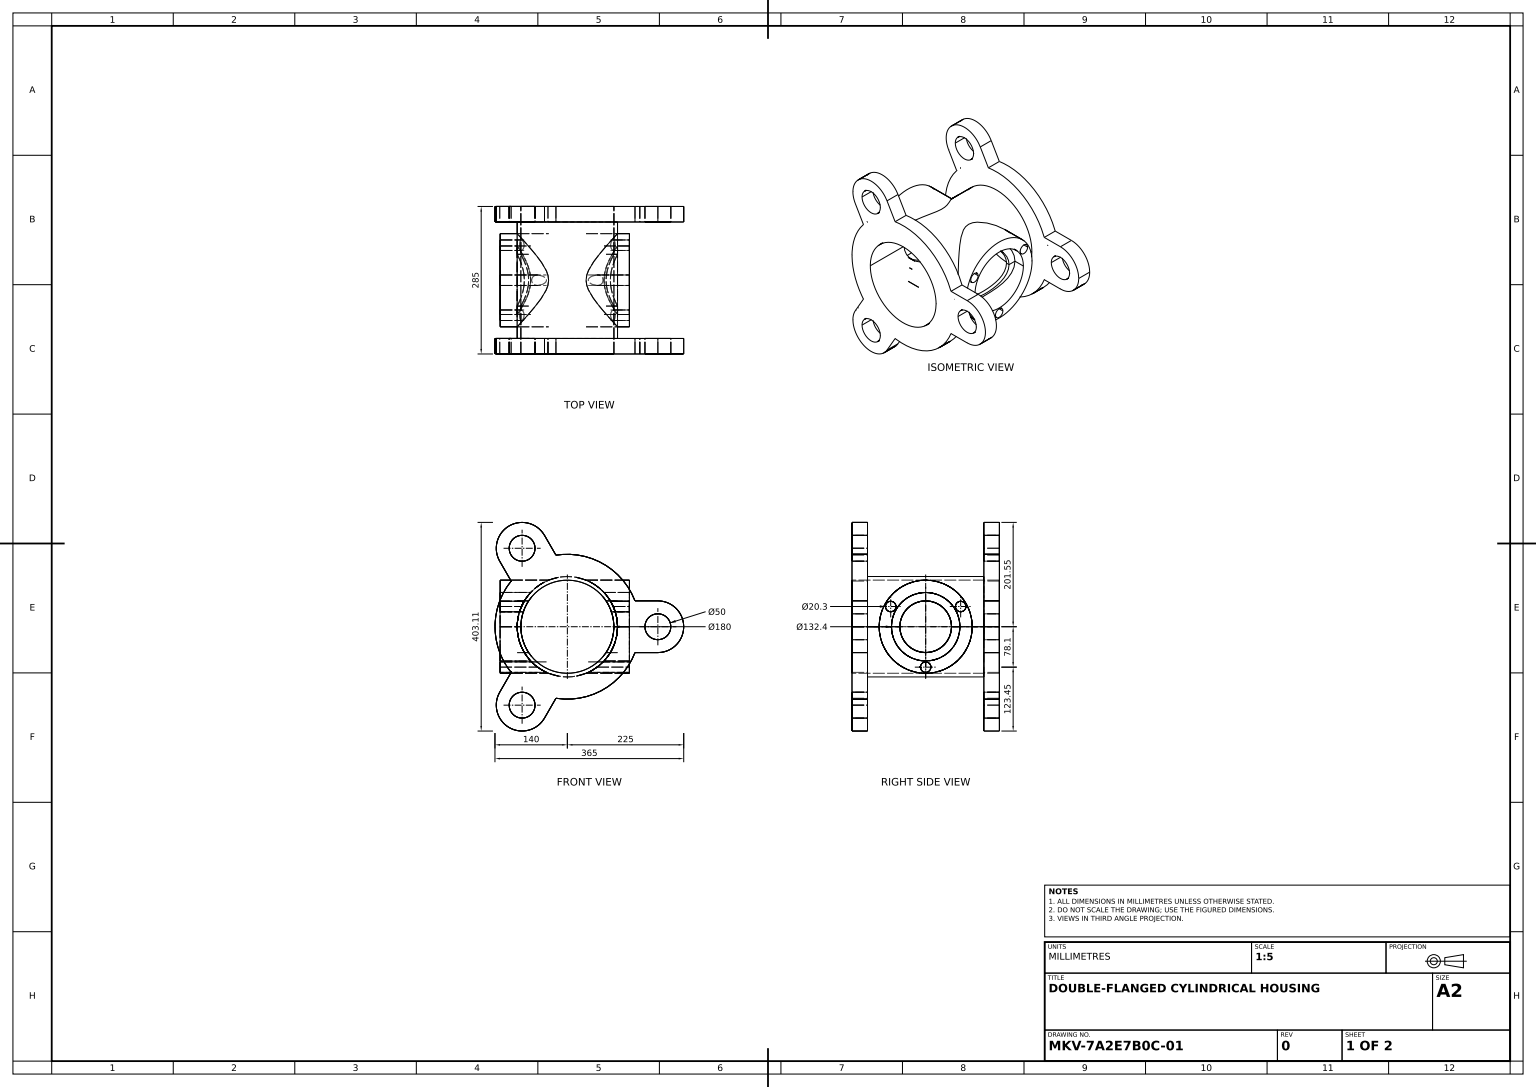
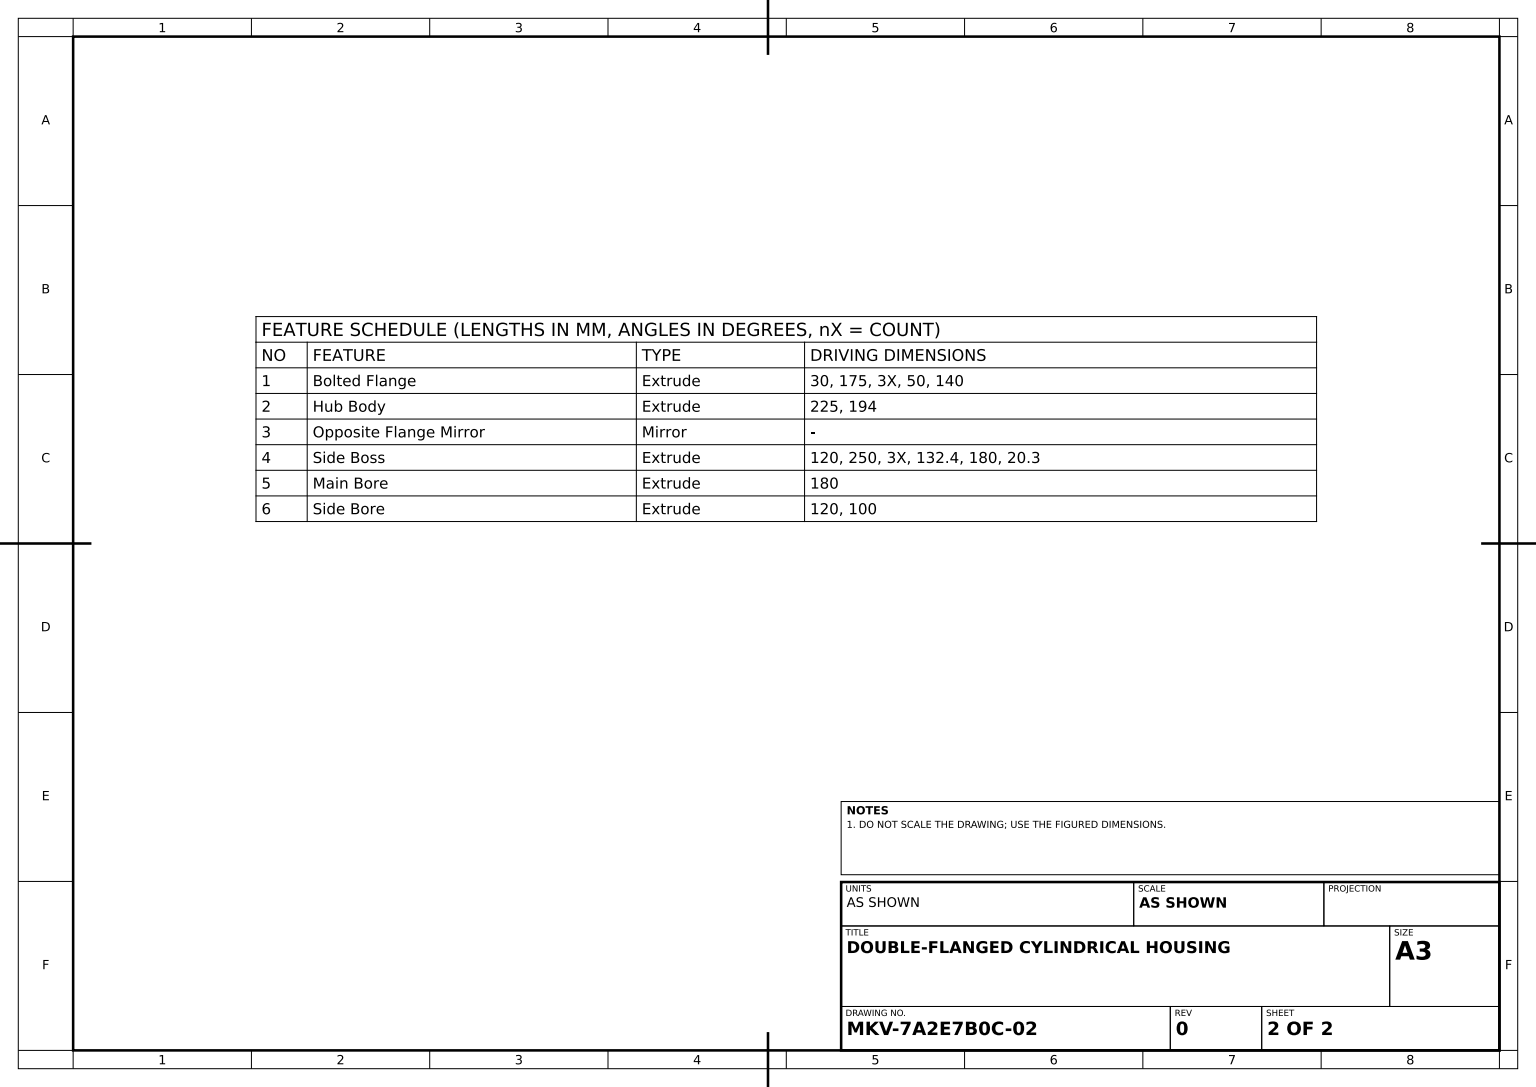
SolidWorks part; units mm, degrees
material "Plain Carbon Steel"
ref_plane "Front Plane" through (0, 0, 0) normal (0, 0, 1) x (1, 0, 0)
ref_plane "Top Plane" through (0, 0, 0) normal (0, 1, 0) x (1, 0, 0)
ref_plane "Right Plane" through (0, 0, 0) normal (1, 0, 0) x (0, 0, -1)
sketch "Flange Profile Sketch" plane through (0, 0, 0) normal (0, 0, 1) x (1, 0, 0)
  line L0 (0, 0) -> (200, 0) construction
  line L1 (0, 0) -> (0, 200) construction
  line L3 (175, 0) -> (175, 200)
  line L4 (175, 50) -> (130.767, 50)
  line L5 (175, -50) -> (130.767, -50)
  line L6 (-130.8013, -126.5544) -> (-108.6848, -88.2475)
  line L7 (-44.1987, -176.5544) -> (-22.0822, -138.2475)
  line L8 (-44.1987, 176.5544) -> (-22.0822, 138.2475)
  line L9 (-130.8013, 126.5544) -> (-108.6848, 88.2475)
  arc A2 (130.767, 50) -> (-22.0822, 138.2475) centre (0, 0) ccw
  arc A4 (175, -50) -> (175, 50) centre (175, 0) ccw
  arc A5 (-130.8013, -126.5544) -> (-44.1987, -176.5544) centre (-87.5, -151.5544) ccw
  arc A6 (-44.1987, 176.5544) -> (-130.8013, 126.5544) centre (-87.5, 151.5544) ccw
  arc A7 (-108.6848, 88.2475) -> (-108.6848, -88.2475) centre (0, 0) ccw
  arc A8 (-22.0822, -138.2475) -> (130.767, -50) centre (0, 0) ccw
  circle A9 centre (175, 0) radius 25
  circle A10 centre (-87.5, -151.5544) radius 25
  circle A11 centre (-87.5, 151.5544) radius 25
  point P23 (0, 0)
  point P28 (0, 0)
  dimension "D1" = 175
  dimension "D2" = 3
  dimension "D3" = 3
  dimension "D4" = 50
  dimension "D5" = 140
  dimension "D6" = 50
extrude "Bolted Flange" add sketch "Flange Profile Sketch" along normal blind 30
sketch "Hub Profile Sketch" plane through (0, 0, 0) normal (0, 0, -1) x (-1, 0, 0)
  circle A0 centre (0, 0) radius 97
  dimension "D1" = 194
extrude "Hub Body" add sketch "Hub Profile Sketch" along normal blind 225
ref_plane "Plane2" through (0, 0, -112.5) normal (0, 0, 1) x (1, 0, 0)
mirror "Opposite Flange Mirror" about plane through (0, 0, -112.5) normal (0, 0, 1) of "Bolted Flange"
ref_plane "Plane3" through (120, 0, 0) normal (1, 0, 0) x (0, 0, -1)
sketch "Side Boss Profile Sketch" plane through (120, 0, 0) normal (1, 0, 0) x (0, 0, -1)
  line L0 (0, 95) -> (225, -95) construction
  line L1 (0, 50) -> (0, 140) construction
  line L2 (225, -50) -> (225, -140) construction
  line L3 (112.5, -66.2) -> (112.5, -90) construction
  circle A0 centre (112.5, 0) radius 90
  circle A1 centre (112.5, 0) radius 66.2
  circle A2 centre (112.5, -78.1) radius 10.15
  circle A3 centre (44.8634, 39.05) radius 10.15
  circle A4 centre (180.1366, 39.05) radius 10.15
  point P20 (112.5, 0)
  dimension "D1" = 3
  dimension "D2" = 20.3
  dimension "D5" = 132.4
  dimension "D6" = 180
extrude "Side Boss" add sketch "Side Boss Profile Sketch" against normal blind 250
sketch "Main Bore Sketch" plane through (0, 0, -255) normal (0, 0, -1) x (-1, 0, 0)
  circle A0 centre (0, 0) radius 90
  dimension "D1" = 180
extrude "Main Bore" cut sketch "Main Bore Sketch" against normal through all
sketch "Side Bore Sketch" plane through (120, 0, 0) normal (1, 0, 0) x (0, 0, -1)
  circle A0 centre (112.5, 0) radius 50
  dimension "D1" = 100
extrude "Side Bore" cut sketch "Side Bore Sketch" against normal through all
